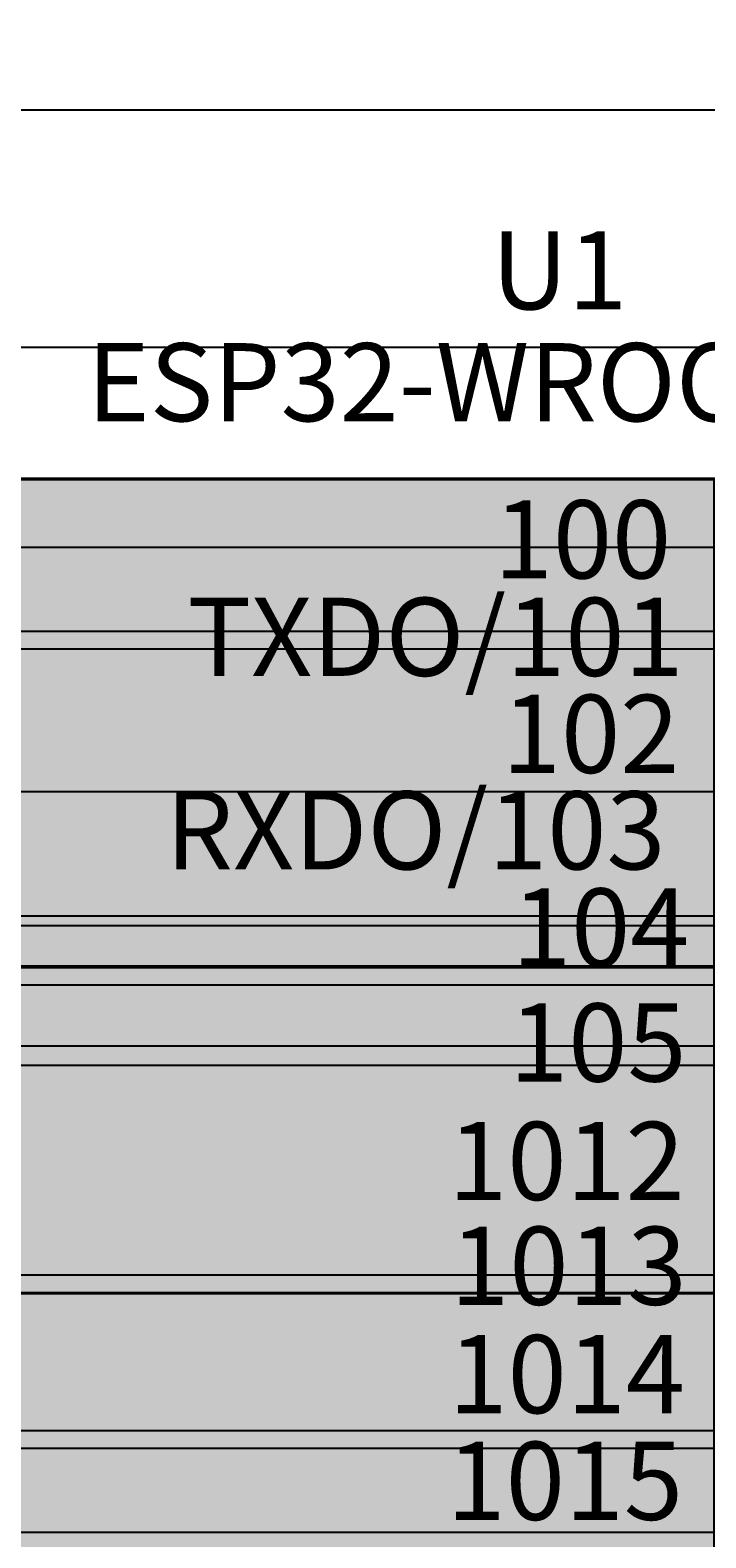
# Model space of a CAD drawing. Units: inches. Extents: x 23 to 132, y 5 to 105.
# Tile 5 of 14: x 66 to 81, y 54 to 87. Entities that reach past the tile are written whole.
import ezdxf

# ---------------------------------------------------------------- set-up
doc = ezdxf.new("R2010")
doc.units = ezdxf.units.IN
doc.header["$MEASUREMENT"] = 0
for name, color, linetype, lineweight in [('A-ANNO-DIMS', 2, 'Continuous', 18), ('E-ANNO-IDEN', 4, 'Continuous', 18), ('E-ANNO-TEXT', 3, 'Continuous', 18), ('E-SYMB', 1, 'Continuous', 35), ('E-SYMB-PATT', 1, 'Continuous', 18)]:
    doc.layers.add(name, color=color, linetype=linetype, lineweight=lineweight)
doc.styles.get("Standard").update_dxf_attribs({"font": 'arial.ttf'})
doc.dimstyles.get("Standard").update_dxf_attribs({"dimtxt": 0.18, "dimasz": 0.18, "dimexe": 0.18, "dimexo": 0.0625, "dimgap": 0.09, "dimtad": 0, "dimtih": 1, "dimtoh": 1, "dimdec": 4, "dimzin": 0, "dimdsep": 46, "dimtxsty": 'Standard', "dimcen": 0.09, "dimadec": 0, "dimazin": 0, "dimtfac": 1, "dimtdec": 4, "dimtofl": 0, "dimtmove": 0, "dimatfit": 3, "dimfxl": 1, "dimtolj": 1, "dimtzin": 0, "dimarcsym": 0})

# ---------------------------------------------------------------- blocks, each defined once
blk = doc.blocks.new('*D2')
at = {"layer": 'A-ANNO-DIMS', "color": 0, "lineweight": -2, "transparency": 16777216}
for p, q in [((28.697, 66.272), (28.697, 105.232)), ((28.877, 105.052), (75.577, 105.052)), ((123.031, 105.052), (76.33, 105.052)), ((123.211, 99.539), (123.211, 105.232))]:
    blk.add_line(p, q, dxfattribs=at)
at = {"layer": 'A-ANNO-DIMS', "color": 0, "transparency": 16777216}
for points in [[(28.877, 105.082), (28.877, 105.022), (28.697, 105.052)], [(123.031, 105.082), (123.031, 105.022), (123.211, 105.052)]]:
    blk.add_solid(points, dxfattribs=at)
at = {"layer": 'Defpoints', "color": 0, "transparency": 16777216}
for p in [(123.211, 105.052), (123.211, 99.477), (28.697, 66.21)]:
    blk.add_point(p, dxfattribs=at)
at = {"layer": 'A-ANNO-DIMS', "color": 0, "transparency": 16777216, "insert": (75.954, 105.052), "char_height": 0.18, "attachment_point": 5}
blk.add_mtext('\\A1;94.51', dxfattribs=at)
blk = doc.blocks.new('*D3')
at = {"layer": 'A-ANNO-DIMS', "color": 0, "lineweight": -2, "transparency": 16777216}
for p, q in [((121.409, 99.285), (129.239, 99.285)), ((129.059, 99.105), (129.059, 55.423)), ((129.059, 11.378), (129.059, 55.06)), ((72.981, 11.198), (129.239, 11.198))]:
    blk.add_line(p, q, dxfattribs=at)
at = {"layer": 'A-ANNO-DIMS', "color": 0, "transparency": 16777216}
for points in [[(129.029, 99.105), (129.089, 99.105), (129.059, 99.285)], [(129.029, 11.378), (129.089, 11.378), (129.059, 11.198)]]:
    blk.add_solid(points, dxfattribs=at)
at = {"layer": 'Defpoints', "color": 0, "transparency": 16777216}
for p in [(121.346, 99.285), (129.059, 99.285), (72.919, 11.198)]:
    blk.add_point(p, dxfattribs=at)
at = {"layer": 'A-ANNO-DIMS', "color": 0, "transparency": 16777216, "insert": (129.059, 55.241), "char_height": 0.18, "attachment_point": 5}
blk.add_mtext('\\A1;88.09', dxfattribs=at)
blk = doc.blocks.new('*D15')
at = {"layer": 'A-ANNO-DIMS', "color": 0, "lineweight": -2, "transparency": 16777216}
for p, q in [((50.327, 77.095), (129.239, 77.095)), ((129.059, 76.915), (129.059, 76.538)), ((129.059, 75.801), (129.059, 76.177)), ((47.783, 75.621), (129.239, 75.621))]:
    blk.add_line(p, q, dxfattribs=at)
at = {"layer": 'A-ANNO-DIMS', "color": 0, "transparency": 16777216}
for points in [[(129.029, 76.915), (129.089, 76.915), (129.059, 77.095)], [(129.029, 75.801), (129.089, 75.801), (129.059, 75.621)]]:
    blk.add_solid(points, dxfattribs=at)
at = {"layer": 'Defpoints', "color": 0, "transparency": 16777216}
for p in [(50.265, 77.095), (47.72, 75.621), (129.059, 75.621)]:
    blk.add_point(p, dxfattribs=at)
at = {"layer": 'A-ANNO-DIMS', "color": 0, "transparency": 16777216, "insert": (129.059, 76.358), "char_height": 0.18, "attachment_point": 5}
blk.add_mtext('\\A1;1.47', dxfattribs=at)
blk = doc.blocks.new('*D16')
at = {"layer": 'A-ANNO-DIMS', "color": 0, "lineweight": -2, "transparency": 16777216}
for p, q in [((47.783, 75.621), (129.239, 75.621)), ((129.059, 75.441), (129.059, 73.177)), ((129.059, 70.55), (129.059, 72.814)), ((47.783, 70.37), (129.239, 70.37))]:
    blk.add_line(p, q, dxfattribs=at)
at = {"layer": 'A-ANNO-DIMS', "color": 0, "transparency": 16777216}
for points in [[(129.029, 75.441), (129.089, 75.441), (129.059, 75.621)], [(129.029, 70.55), (129.089, 70.55), (129.059, 70.37)]]:
    blk.add_solid(points, dxfattribs=at)
at = {"layer": 'Defpoints', "color": 0, "transparency": 16777216}
for p in [(47.72, 75.621), (47.72, 70.37), (129.059, 70.37)]:
    blk.add_point(p, dxfattribs=at)
at = {"layer": 'A-ANNO-DIMS', "color": 0, "transparency": 16777216, "insert": (129.059, 72.996), "char_height": 0.18, "attachment_point": 5}
blk.add_mtext('\\A1;5.25', dxfattribs=at)
blk = doc.blocks.new('*D17')
at = {"layer": 'A-ANNO-DIMS', "color": 0, "lineweight": -2, "transparency": 16777216}
for p, q in [((47.783, 70.37), (129.239, 70.37)), ((129.059, 70.19), (129.059, 68.678)), ((129.059, 66.801), (129.059, 68.314)), ((47.783, 66.621), (129.239, 66.621))]:
    blk.add_line(p, q, dxfattribs=at)
at = {"layer": 'A-ANNO-DIMS', "color": 0, "transparency": 16777216}
for points in [[(129.029, 70.19), (129.089, 70.19), (129.059, 70.37)], [(129.029, 66.801), (129.089, 66.801), (129.059, 66.621)]]:
    blk.add_solid(points, dxfattribs=at)
at = {"layer": 'Defpoints', "color": 0, "transparency": 16777216}
for p in [(47.72, 70.37), (47.72, 66.621), (129.059, 66.621)]:
    blk.add_point(p, dxfattribs=at)
at = {"layer": 'A-ANNO-DIMS', "color": 0, "transparency": 16777216, "insert": (129.059, 68.496), "char_height": 0.18, "attachment_point": 5}
blk.add_mtext('\\A1;3.75', dxfattribs=at)
blk = doc.blocks.new('*D57')
at = {"layer": 'A-ANNO-DIMS', "color": 0, "lineweight": -2, "transparency": 16777216}
for p, q in [((30.358, 64.901), (129.239, 64.901)), ((129.059, 64.721), (129.059, 62.62)), ((129.059, 60.155), (129.059, 62.256)), ((30.358, 59.975), (129.239, 59.975))]:
    blk.add_line(p, q, dxfattribs=at)
at = {"layer": 'A-ANNO-DIMS', "color": 0, "transparency": 16777216}
for points in [[(129.029, 64.721), (129.089, 64.721), (129.059, 64.901)], [(129.029, 60.155), (129.089, 60.155), (129.059, 59.975)]]:
    blk.add_solid(points, dxfattribs=at)
at = {"layer": 'Defpoints', "color": 0, "transparency": 16777216}
for p in [(30.295, 64.901), (129.059, 64.901), (30.295, 59.975)]:
    blk.add_point(p, dxfattribs=at)
at = {"layer": 'A-ANNO-DIMS', "color": 0, "transparency": 16777216, "insert": (129.059, 62.438), "char_height": 0.18, "attachment_point": 5}
blk.add_mtext('\\A1;4.925', dxfattribs=at)
blk = doc.blocks.new('*D58')
at = {"layer": 'A-ANNO-DIMS', "color": 0, "lineweight": -2, "transparency": 16777216}
for p, q in [((30.358, 73.814), (129.239, 73.814)), ((129.059, 73.634), (129.059, 70.194)), ((129.059, 66.39), (129.059, 69.83)), ((30.359, 66.21), (129.239, 66.21))]:
    blk.add_line(p, q, dxfattribs=at)
at = {"layer": 'A-ANNO-DIMS', "color": 0, "transparency": 16777216}
for points in [[(129.029, 73.634), (129.089, 73.634), (129.059, 73.814)], [(129.029, 66.39), (129.089, 66.39), (129.059, 66.21)]]:
    blk.add_solid(points, dxfattribs=at)
at = {"layer": 'Defpoints', "color": 0, "transparency": 16777216}
for p in [(30.295, 73.814), (129.059, 73.814), (30.297, 66.21)]:
    blk.add_point(p, dxfattribs=at)
at = {"layer": 'A-ANNO-DIMS', "color": 0, "transparency": 16777216, "insert": (129.059, 70.012), "char_height": 0.18, "attachment_point": 5}
blk.add_mtext('\\A1;7.604', dxfattribs=at)
blk = doc.blocks.new('*D65')
at = {"layer": 'A-ANNO-DIMS', "color": 0, "lineweight": -2, "transparency": 16777216}
for p, q in [((38.414, 67.485), (129.239, 67.485)), ((129.059, 67.305), (129.059, 66.165)), ((129.059, 64.66), (129.059, 65.801)), ((38.414, 64.48), (129.239, 64.48))]:
    blk.add_line(p, q, dxfattribs=at)
at = {"layer": 'A-ANNO-DIMS', "color": 0, "transparency": 16777216}
for points in [[(129.029, 67.305), (129.089, 67.305), (129.059, 67.485)], [(129.029, 64.66), (129.089, 64.66), (129.059, 64.48)]]:
    blk.add_solid(points, dxfattribs=at)
at = {"layer": 'Defpoints', "color": 0, "transparency": 16777216}
for p in [(38.351, 67.485), (129.059, 67.485), (38.351, 64.48)]:
    blk.add_point(p, dxfattribs=at)
at = {"layer": 'A-ANNO-DIMS', "color": 0, "transparency": 16777216, "insert": (129.059, 65.983), "char_height": 0.18, "attachment_point": 5}
blk.add_mtext('\\A1;3.005', dxfattribs=at)
blk = doc.blocks.new('*D70')
at = {"layer": 'A-ANNO-DIMS', "color": 0, "lineweight": -2, "transparency": 16777216}
for p, q in [((35.392, 56.625), (129.239, 56.625)), ((129.059, 56.445), (129.059, 55.716)), ((129.059, 54.624), (129.059, 55.352)), ((33.892, 54.444), (129.239, 54.444))]:
    blk.add_line(p, q, dxfattribs=at)
at = {"layer": 'A-ANNO-DIMS', "color": 0, "transparency": 16777216}
for points in [[(129.029, 56.445), (129.089, 56.445), (129.059, 56.625)], [(129.029, 54.624), (129.089, 54.624), (129.059, 54.444)]]:
    blk.add_solid(points, dxfattribs=at)
at = {"layer": 'Defpoints', "color": 0, "transparency": 16777216}
for p in [(35.33, 56.625), (33.83, 54.444), (129.059, 54.444)]:
    blk.add_point(p, dxfattribs=at)
at = {"layer": 'A-ANNO-DIMS', "color": 0, "transparency": 16777216, "insert": (129.059, 55.534), "char_height": 0.18, "attachment_point": 5}
blk.add_mtext('\\A1;2.18', dxfattribs=at)
blk = doc.blocks.new('*D78')
at = {"layer": 'A-ANNO-DIMS', "color": 0, "lineweight": -2, "transparency": 16777216}
for p, q in [((112.773, 67.688), (22.942, 67.688)), ((23.122, 67.508), (23.122, 67.314)), ((23.122, 66.759), (23.122, 66.953)), ((112.773, 66.579), (22.942, 66.579))]:
    blk.add_line(p, q, dxfattribs=at)
at = {"layer": 'A-ANNO-DIMS', "color": 0, "transparency": 16777216}
for points in [[(23.092, 67.508), (23.152, 67.508), (23.122, 67.688)], [(23.092, 66.759), (23.152, 66.759), (23.122, 66.579)]]:
    blk.add_solid(points, dxfattribs=at)
at = {"layer": 'Defpoints', "color": 0, "transparency": 16777216}
for p in [(23.122, 67.688), (112.835, 67.688), (112.835, 66.579)]:
    blk.add_point(p, dxfattribs=at)
at = {"layer": 'A-ANNO-DIMS', "color": 0, "transparency": 16777216, "insert": (23.122, 67.133), "char_height": 0.18, "attachment_point": 5}
blk.add_mtext('\\A1;1.11', dxfattribs=at)
blk = doc.blocks.new('*D79')
at = {"layer": 'A-ANNO-DIMS', "color": 0, "lineweight": -2, "transparency": 16777216}
for p, q in [((114.373, 66.579), (22.942, 66.579)), ((23.122, 66.399), (23.122, 63.267)), ((23.122, 59.77), (23.122, 62.903)), ((114.371, 59.59), (22.942, 59.59))]:
    blk.add_line(p, q, dxfattribs=at)
at = {"layer": 'A-ANNO-DIMS', "color": 0, "transparency": 16777216}
for points in [[(23.092, 66.399), (23.152, 66.399), (23.122, 66.579)], [(23.092, 59.77), (23.152, 59.77), (23.122, 59.59)]]:
    blk.add_solid(points, dxfattribs=at)
at = {"layer": 'Defpoints', "color": 0, "transparency": 16777216}
for p in [(23.122, 66.579), (114.435, 66.579), (114.434, 59.59)]:
    blk.add_point(p, dxfattribs=at)
at = {"layer": 'A-ANNO-DIMS', "color": 0, "transparency": 16777216, "insert": (23.122, 63.085), "char_height": 0.18, "attachment_point": 5}
blk.add_mtext('\\A1;6.988', dxfattribs=at)
blk = doc.blocks.new('*D80')
at = {"layer": 'A-ANNO-DIMS', "color": 0, "lineweight": -2, "transparency": 16777216}
for p, q in [((114.373, 73.429), (22.942, 73.429)), ((23.122, 73.249), (23.122, 70.741)), ((23.122, 67.868), (23.122, 70.377)), ((114.373, 67.688), (22.942, 67.688))]:
    blk.add_line(p, q, dxfattribs=at)
at = {"layer": 'A-ANNO-DIMS', "color": 0, "transparency": 16777216}
for points in [[(23.092, 73.249), (23.152, 73.249), (23.122, 73.429)], [(23.092, 67.868), (23.152, 67.868), (23.122, 67.688)]]:
    blk.add_solid(points, dxfattribs=at)
at = {"layer": 'Defpoints', "color": 0, "transparency": 16777216}
for p in [(23.122, 73.429), (114.435, 73.429), (114.435, 67.688)]:
    blk.add_point(p, dxfattribs=at)
at = {"layer": 'A-ANNO-DIMS', "color": 0, "transparency": 16777216, "insert": (23.122, 70.559), "char_height": 0.18, "attachment_point": 5}
blk.add_mtext('\\A1;5.741', dxfattribs=at)
blk = doc.blocks.new('*D81')
at = {"layer": 'A-ANNO-DIMS', "color": 0, "lineweight": -2, "transparency": 16777216}
for p, q in [((110.705, 59.566), (22.942, 59.566)), ((23.122, 59.386), (23.122, 58.085)), ((23.122, 56.42), (23.122, 57.721)), ((110.759, 56.24), (22.942, 56.24))]:
    blk.add_line(p, q, dxfattribs=at)
at = {"layer": 'A-ANNO-DIMS', "color": 0, "transparency": 16777216}
for points in [[(23.092, 59.386), (23.152, 59.386), (23.122, 59.566)], [(23.092, 56.42), (23.152, 56.42), (23.122, 56.24)]]:
    blk.add_solid(points, dxfattribs=at)
at = {"layer": 'Defpoints', "color": 0, "transparency": 16777216}
for p in [(23.122, 59.566), (110.768, 59.566), (110.822, 56.24)]:
    blk.add_point(p, dxfattribs=at)
at = {"layer": 'A-ANNO-DIMS', "color": 0, "transparency": 16777216, "insert": (23.122, 57.903), "char_height": 0.18, "attachment_point": 5}
blk.add_mtext('\\A1;3.326', dxfattribs=at)
blk = doc.blocks.new('*D85')
at = {"layer": 'A-ANNO-DIMS', "color": 0, "lineweight": -2, "transparency": 16777216}
for p, q in [((106.903, 97.776), (22.942, 97.776)), ((23.122, 97.596), (23.122, 87.606)), ((23.122, 77.251), (23.122, 87.242)), ((106.964, 77.071), (22.942, 77.071))]:
    blk.add_line(p, q, dxfattribs=at)
at = {"layer": 'A-ANNO-DIMS', "color": 0, "transparency": 16777216}
for points in [[(23.092, 97.596), (23.152, 97.596), (23.122, 97.776)], [(23.092, 77.251), (23.152, 77.251), (23.122, 77.071)]]:
    blk.add_solid(points, dxfattribs=at)
at = {"layer": 'Defpoints', "color": 0, "transparency": 16777216}
for p in [(23.122, 97.776), (106.965, 97.776), (107.026, 77.071)]:
    blk.add_point(p, dxfattribs=at)
at = {"layer": 'A-ANNO-DIMS', "color": 0, "transparency": 16777216, "insert": (23.122, 87.424), "char_height": 0.18, "attachment_point": 5}
blk.add_mtext('\\A1;20.705', dxfattribs=at)
blk = doc.blocks.new('*D86')
at = {"layer": 'A-ANNO-DIMS', "color": 0, "lineweight": -2, "transparency": 16777216}
for p, q in [((110.027, 79.916), (22.942, 79.916)), ((23.122, 79.736), (23.122, 78.675)), ((23.122, 77.251), (23.122, 78.312)), ((106.964, 77.071), (22.942, 77.071))]:
    blk.add_line(p, q, dxfattribs=at)
at = {"layer": 'A-ANNO-DIMS', "color": 0, "transparency": 16777216}
for points in [[(23.092, 79.736), (23.152, 79.736), (23.122, 79.916)], [(23.092, 77.251), (23.152, 77.251), (23.122, 77.071)]]:
    blk.add_solid(points, dxfattribs=at)
at = {"layer": 'Defpoints', "color": 0, "transparency": 16777216}
for p in [(23.122, 79.916), (110.089, 79.916), (107.026, 77.071)]:
    blk.add_point(p, dxfattribs=at)
at = {"layer": 'A-ANNO-DIMS', "color": 0, "transparency": 16777216, "insert": (23.122, 78.493), "char_height": 0.18, "attachment_point": 5}
blk.add_mtext('\\A1;2.84', dxfattribs=at)
blk = doc.blocks.new('*D87')
at = {"layer": 'A-ANNO-DIMS', "color": 0, "lineweight": -2, "transparency": 16777216}
for p, q in [((110.027, 85.021), (22.942, 85.021)), ((23.122, 84.841), (23.122, 82.65)), ((23.122, 80.096), (23.122, 82.286)), ((110.027, 79.916), (22.942, 79.916))]:
    blk.add_line(p, q, dxfattribs=at)
at = {"layer": 'A-ANNO-DIMS', "color": 0, "transparency": 16777216}
for points in [[(23.092, 84.841), (23.152, 84.841), (23.122, 85.021)], [(23.092, 80.096), (23.152, 80.096), (23.122, 79.916)]]:
    blk.add_solid(points, dxfattribs=at)
at = {"layer": 'Defpoints', "color": 0, "transparency": 16777216}
for p in [(23.122, 85.021), (110.089, 85.021), (110.089, 79.916)]:
    blk.add_point(p, dxfattribs=at)
at = {"layer": 'A-ANNO-DIMS', "color": 0, "transparency": 16777216, "insert": (23.122, 82.468), "char_height": 0.18, "attachment_point": 5}
blk.add_mtext('\\A1;5.105', dxfattribs=at)
blk = doc.blocks.new('*D88')
at = {"layer": 'A-ANNO-DIMS', "color": 0, "lineweight": -2, "transparency": 16777216}
for p, q in [((110.027, 89.722), (22.942, 89.722)), ((23.122, 89.542), (23.122, 87.554)), ((23.122, 85.201), (23.122, 87.19)), ((110.027, 85.021), (22.942, 85.021))]:
    blk.add_line(p, q, dxfattribs=at)
at = {"layer": 'A-ANNO-DIMS', "color": 0, "transparency": 16777216}
for points in [[(23.092, 89.542), (23.152, 89.542), (23.122, 89.722)], [(23.092, 85.201), (23.152, 85.201), (23.122, 85.021)]]:
    blk.add_solid(points, dxfattribs=at)
at = {"layer": 'Defpoints', "color": 0, "transparency": 16777216}
for p in [(23.122, 89.722), (110.089, 89.722), (110.089, 85.021)]:
    blk.add_point(p, dxfattribs=at)
at = {"layer": 'A-ANNO-DIMS', "color": 0, "transparency": 16777216, "insert": (23.122, 87.372), "char_height": 0.18, "attachment_point": 5}
blk.add_mtext('\\A1;4.702', dxfattribs=at)

msp = doc.modelspace()

# ---------------------------------------------------------------- hatches: boundary and pattern name
at = {"layer": 'E-SYMB-PATT'}
h = msp.add_hatch(color=256, dxfattribs=at)
h.dxf.hatch_style = 1
h.paths.add_polyline_path([(80.9692, 77.095), (50.2646, 77.095), (50.2646, 18.0066), (80.9692, 18.0066)])

# ---------------------------------------------------------------- linework, layer by layer
at = {"layer": 'E-SYMB'}
msp.add_lwpolyline([(50.2646, 77.095), (80.9692, 77.095), (80.9692, 18.0066), (50.2646, 18.0066)], close=True, dxfattribs=at)

# ---------------------------------------------------------------- texts
at = {"layer": 'E-ANNO-IDEN'}
for s, height, p in [('U1', 1.67943, (76.1717, 80.7355)), ('ESP32-WROOM-32', 1.679435, (67.4727, 78.3292))]:
    msp.add_text(s, height=height, dxfattribs=at).set_placement(p)
at = {"layer": 'E-ANNO-TEXT'}
for s, p in [('100', (76.2261, 74.9502)), ('TXDO/101', (69.6323, 72.8539)), ('102', (76.4012, 70.7682)), ('RXDO/103', (69.1621, 68.6931)), ('104', (76.6173, 66.6033)), ('105', (76.5565, 64.1306)), ('1012', (75.2445, 61.585)), ('1013', (75.2882, 59.3297)), ('1014', (75.251, 56.9997)), ('1015', (75.2104, 54.7052))]:
    msp.add_text(s, height=1.67943, dxfattribs=at).set_placement(p)

# ---------------------------------------------------------------- dimensions: what is measured, and where the dimension line sits
at = {"layer": 'A-ANNO-DIMS'}
dim = msp.add_linear_dim(base=(123.2107, 105.052), p1=(28.6965, 66.2099), p2=(123.2107, 99.477), dimstyle='Standard', override={"dimdec": 2, "dimlfac": 1, "dimrnd": 0, "dimzin": 0, "dimdsep": 46, "dimlunit": 2}, dxfattribs=at)
dim.commit()
dim.dimension.update_dxf_attribs({"geometry": '*D2', "text_midpoint": (75.9536, 105.052)})
for base, p1, p2, override, picture, middle in [((129.0589, 99.2846), (72.9188, 11.1983), (121.3461, 99.2846), {"dimdec": 2, "dimlfac": 1, "dimrnd": 0, "dimzin": 0, "dimdsep": 46, "dimlunit": 2}, '*D3', (129.0589, 55.2415)), ((23.1215, 97.7764), (107.026, 77.0711), (106.9652, 97.7764), {"dimdec": 3, "dimlfac": 1, "dimrnd": 0, "dimzin": 0, "dimdsep": 46, "dimlunit": 2}, '*D85', (23.1215, 87.4238)), ((23.12152, 89.7224), (110.08916, 85.02085), (110.08916, 89.7224), {"dimdec": 3, "dimlfac": 1, "dimrnd": 0, "dimzin": 0, "dimdsep": 46, "dimlunit": 2}, '*D88', (23.12152, 87.37162)), ((23.1215, 85.0209), (110.0892, 79.9158), (110.0892, 85.0209), {"dimdec": 3, "dimlfac": 1, "dimrnd": 0, "dimzin": 0, "dimdsep": 46, "dimlunit": 2}, '*D87', (23.1215, 82.4683)), ((23.1215, 79.9158), (107.026, 77.0711), (110.0892, 79.9158), {"dimdec": 2, "dimlfac": 1, "dimrnd": 0, "dimzin": 0, "dimdsep": 46, "dimlunit": 2}, '*D86', (23.1215, 78.4935)), ((129.0589, 75.6207), (50.2646, 77.095), (47.7202, 75.6207), {"dimdec": 2, "dimlfac": 1, "dimrnd": 0, "dimzin": 0, "dimdsep": 46, "dimlunit": 2}, '*D15', (129.0589, 76.3579)), ((129.0589, 70.3705), (47.7202, 75.6207), (47.7202, 70.3705), {"dimdec": 2, "dimlfac": 1, "dimrnd": 0, "dimzin": 0, "dimdsep": 46, "dimlunit": 2}, '*D16', (129.0589, 72.9956)), ((129.05891, 73.81438), (30.29652, 66.20989), (30.29537, 73.81438), {"dimdec": 3, "dimlfac": 1, "dimrnd": 0, "dimzin": 0, "dimdsep": 46, "dimlunit": 2}, '*D58', (129.05891, 70.01213)), ((23.1215, 73.4293), (114.4351, 67.6881), (114.4351, 73.4293), {"dimdec": 3, "dimlfac": 1, "dimrnd": 0, "dimzin": 0, "dimdsep": 46, "dimlunit": 2}, '*D80', (23.1215, 70.5587)), ((129.0589, 66.621), (47.7202, 70.3705), (47.7202, 66.621), {"dimdec": 2, "dimlfac": 1, "dimrnd": 0, "dimzin": 0, "dimdsep": 46, "dimlunit": 2}, '*D17', (129.0589, 68.4957)), ((23.1215, 67.6881), (112.8351, 66.5788), (112.8351, 67.6881), {"dimdec": 2, "dimlfac": 1, "dimrnd": 0, "dimzin": 0, "dimdsep": 46, "dimlunit": 2}, '*D78', (23.1215, 67.1334)), ((129.0589, 67.4851), (38.3512, 64.4801), (38.3512, 67.4851), {"dimdec": 3, "dimlfac": 1, "dimrnd": 0, "dimzin": 0, "dimdsep": 46, "dimlunit": 2}, '*D65', (129.0589, 65.9826)), ((23.1215, 66.5788), (114.434, 59.5904), (114.4351, 66.5788), {"dimdec": 3, "dimlfac": 1, "dimrnd": 0, "dimzin": 0, "dimdsep": 46, "dimlunit": 2}, '*D79', (23.1215, 63.0846)), ((129.0589, 64.9007), (30.2954, 59.9755), (30.2954, 64.9007), {"dimdec": 3, "dimlfac": 1, "dimrnd": 0, "dimzin": 0, "dimdsep": 46, "dimlunit": 2}, '*D57', (129.0589, 62.4381)), ((23.1215, 59.566), (110.8219, 56.2399), (110.7677, 59.566), {"dimdec": 3, "dimlfac": 1, "dimrnd": 0, "dimzin": 0, "dimdsep": 46, "dimlunit": 2}, '*D81', (23.1215, 57.9029)), ((129.0589, 54.4437), (35.3299, 56.6249), (33.8299, 54.4437), {"dimdec": 2, "dimlfac": 1, "dimrnd": 0, "dimzin": 0, "dimdsep": 46, "dimlunit": 2}, '*D70', (129.0589, 55.5343))]:
    dim = msp.add_linear_dim(base=base, p1=p1, p2=p2, angle=90, dimstyle='Standard', override=override, dxfattribs=at)
    dim.commit()
    dim.dimension.update_dxf_attribs({"geometry": picture, "text_midpoint": middle})

doc.saveas('drawing.dxf')
